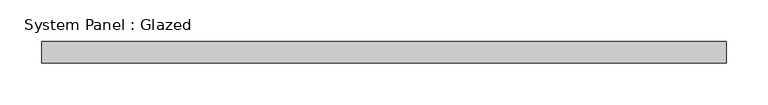
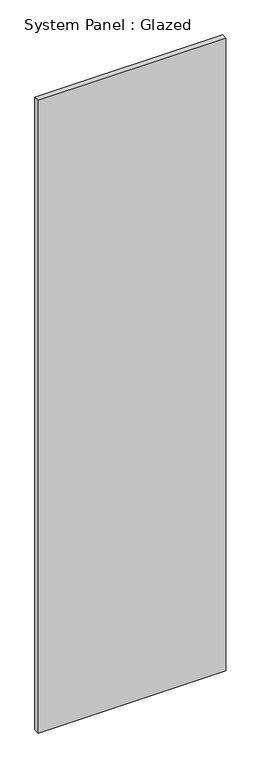
"""IFC4 building model written with IfcOpenShell, lengths in millimetres: plate geometry, System Panel : Glazed."""

from ifc_helpers import new_model, si_unit, origin, origin_with_axes, place, context, project, spatial, polyline, outline, extrude, source, transform, mapped, element, save


def system_panel_glazed_52d31088(model_context):
    return source(origin(), model_context, "Body", "SweptSolid", [
        extrude(outline(polyline([(409.575, 19.05), (-409.575, 19.05), (-409.575, 44.45), (409.575, 44.45), (409.575, 19.05)])), origin_with_axes(), (0.0, 0.0, 1.0), 2921.0),
    ])


if __name__ == "__main__":
    model = new_model("IFC4")
    model_context = context("Model", 3, world=origin())
    ifc_project = project(units=[si_unit("LENGTHUNIT", "METRE", prefix="MILLI")], contexts=[model_context])
    site = spatial("IfcSite", under=ifc_project)
    building = spatial("IfcBuilding", under=site)
    placement = place(None, origin())
    system_panel_glazed_shape = system_panel_glazed_52d31088(model_context)
    element("IfcPlate", 1, ObjectType="System Panel : Glazed", at=placement, inside=building, context=model_context, shape_type="MappedRepresentation", body=[
        mapped(system_panel_glazed_shape, transform((0.0, 0.0, 0.0), x_axis=(1.0, 0.0, 0.0), y_axis=(0.0, 1.0, 0.0), z_axis=(0.0, 0.0, 1.0))),
    ])
    save(model, "model.ifc")

# Revit data of these elements
# Type "System Panel : Glazed"
#   Construction Type Id = "GSP4R"
#   Analytic Construction = "1/8 in Pilkington single glazing"
#   Visual Light Transmittance = 0.9
#   Solar Heat Gain Coefficient = 0.86
#   Heat Transfer Coefficient (U) = 1.18115 BTU/(h·ft²·°F)
#   Define Thermal Properties by = 1
# Element 1 (IfcPlate, "System Panel : Glazed")
#   Materials on its faces: "Glass"
# Materials
#   "Glass": class "Glass", colour RGB 0 128 192, transparency 0.75, Description = "Soda Lime Glass", Cost = 0
